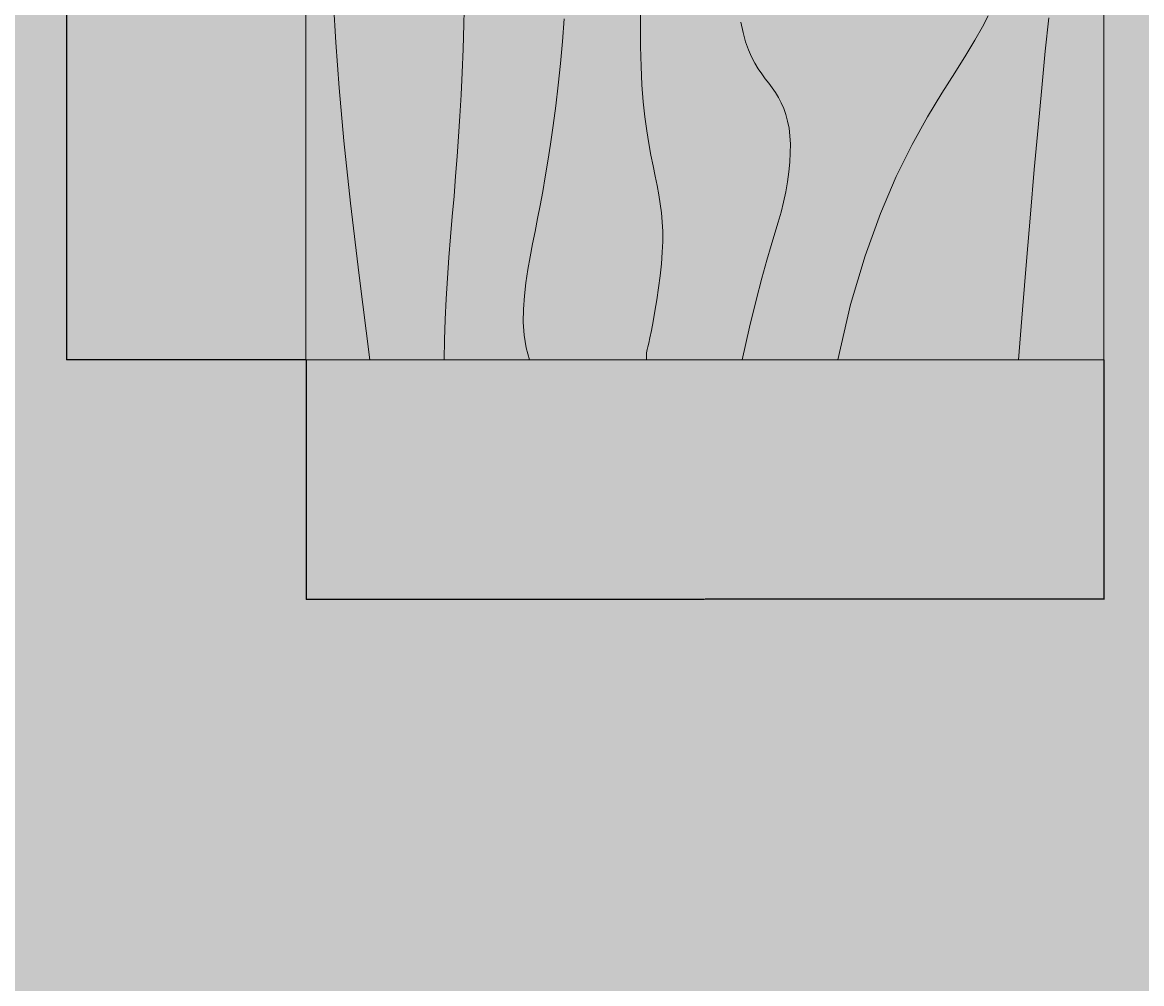
# Model space of a CAD drawing. Units: millimetres. Extents: x -229 to 16545, y -10488 to 4272.
# Tile 15 of 29: x 11804 to 12629, y -4126 to -3417. Entities that reach past the tile are written whole.
import ezdxf

# ---------------------------------------------------------------- set-up
doc = ezdxf.new("R2010")
doc.units = ezdxf.units.MM
for name, color, linetype, lineweight in [('A-ANNO-DIMS', 2, 'Continuous', 18), ('A-FURN', 8, 'Continuous', 18), ('A-FURN-PATT', 252, 'Continuous', 13)]:
    doc.layers.add(name, color=color, linetype=linetype, lineweight=lineweight)
doc.layers.add('A-FLOR-PATT', color=254, linetype='Continuous', lineweight=13, true_color=0xfeeab9)
doc.styles.get("Standard").update_dxf_attribs({"font": 'arial.ttf'})
doc.dimstyles.get("Standard").update_dxf_attribs({"dimtxt": 0.18, "dimasz": 0.18, "dimexe": 0.18, "dimexo": 0.0625, "dimgap": 0.09, "dimtad": 0, "dimtih": 1, "dimtoh": 1, "dimdec": 4, "dimzin": 0, "dimdsep": 46, "dimtxsty": 'Standard', "dimcen": 0.09, "dimadec": 0, "dimazin": 0, "dimtfac": 1, "dimtdec": 4, "dimtofl": 0, "dimtmove": 0, "dimatfit": 3, "dimfxl": 1, "dimtolj": 1, "dimtzin": 0, "dimarcsym": 0})

# ---------------------------------------------------------------- blocks, each defined once
blk = doc.blocks.new('Table - Rectangular Woodgrain 60 x 30 in.')
for p, q in [((60, 0), (0, 0)), ((60, -30), (60, 0)), ((0, -30), (60, -30))]:
    blk.add_line(p, q)
for points in [[(47.1333, -2.0667), (48.3862, -2.1947), (49.7625, -2.3281), (51.2513, -2.4663), (52.8416, -2.6083), (54.5226, -2.7535), (56.2833, -2.9011), (58.1127, -3.0501), (60, -3.2)], [(47.0542, -4.3417), (47.4756, -4.5629), (47.9661, -4.8427), (48.5372, -5.1866), (49.2, -5.6), (49.9676, -6.0844), (50.8594, -6.625), (51.8965, -7.2031), (53.1, -7.8), (54.491, -8.3969), (56.0906, -8.975), (57.9199, -9.5156), (60, -10)], [(47.2906, -13.6417), (47.6858, -13.5604), (48.0333, -13.4667), (48.3375, -13.3608), (48.6042, -13.2448), (48.8396, -13.121), (49.05, -12.9917), (49.2417, -12.8593), (49.4208, -12.7261), (49.5937, -12.5944), (49.7667, -12.4667), (49.9452, -12.3451), (50.1323, -12.2313), (50.3303, -12.1268), (50.5416, -12.0333), (50.7686, -11.9524), (51.0135, -11.8854), (51.2788, -11.8341), (51.5666, -11.8), (51.8785, -11.7843), (52.2116, -11.7865), (52.562, -11.8059), (52.926, -11.8417), (53.2998, -11.8931), (53.6795, -11.9594), (54.0614, -12.0397), (54.4416, -12.1333), (54.8223, -12.2401), (55.2293, -12.3625), (55.6942, -12.5037), (56.2489, -12.6667), (56.9251, -12.8547), (57.7545, -13.0708), (58.7689, -13.3182), (60, -13.6)], [(46.4858, -17.4012), (47.3802, -17.4156), (48.2074, -17.416), (48.9667, -17.4), (49.6583, -17.3662), (50.2872, -17.3167), (50.8595, -17.2547), (51.3812, -17.1833), (51.8584, -17.1057), (52.2971, -17.025), (52.7034, -16.9443), (53.0833, -16.8667), (53.443, -16.7951), (53.789, -16.7313), (54.128, -16.6768), (54.4666, -16.6334), (54.8115, -16.6024), (55.1693, -16.5854), (55.5465, -16.5841), (55.95, -16.6), (56.3828, -16.6337), (56.8346, -16.6823), (57.2915, -16.7418), (57.7396, -16.8084), (58.165, -16.878), (58.5539, -16.9469), (58.8924, -17.0111), (59.1666, -17.0667), (59.3679, -17.1107), (59.5078, -17.1438), (59.6032, -17.1675), (59.6708, -17.1833), (59.7275, -17.193), (59.7901, -17.1979), (59.8753, -17.1998), (60, -17.2)], [(47.1747, -20.2844), (48.0163, -20.3488), (48.8479, -20.425), (49.66, -20.5106), (50.4429, -20.6031), (51.1872, -20.7004), (51.8833, -20.8), (52.5246, -20.8999), (53.1166, -20.9995), (53.6681, -21.0983), (54.1875, -21.1958), (54.6834, -21.2919), (55.1646, -21.3859), (55.6394, -21.4777), (56.1167, -21.5667), (56.6028, -21.6515), (57.0961, -21.7266), (57.5929, -21.7852), (58.0896, -21.8208), (58.5823, -21.8268), (59.0674, -21.7964), (59.5412, -21.723), (60, -21.6)], [(46.3557, -24.0451), (47.3667, -24.0667), (48.309, -24.0947), (49.1928, -24.1287), (50.0284, -24.168), (50.826, -24.2125), (51.5959, -24.2617), (52.3483, -24.3151), (53.0935, -24.3725), (53.8417, -24.4334), (54.6009, -24.497), (55.3699, -24.561), (56.1454, -24.6226), (56.9239, -24.6792), (57.7021, -24.7279), (58.4764, -24.7662), (59.2435, -24.7911), (60, -24.8)], [(46.5843, -28.9641), (48.0579, -28.8816), (49.7666, -28.7542), (51.7629, -28.5721), (54.0989, -28.3255), (56.8272, -28.0048), (60, -27.6)]]:
    blk.add_lwpolyline(points)
blk = doc.blocks.new('*D41')
at = {"layer": 'A-ANNO-DIMS', "color": 0, "lineweight": -2, "transparency": 16777216}
for p, q in [((12012.63, -2489.42), (11836.03, -2489.42)), ((11836.21, -2489.6), (11836.21, -3077.54)), ((11836.21, -3665.84), (11836.21, -3077.9)), ((12012.63, -3666.02), (11836.03, -3666.02))]:
    blk.add_line(p, q, dxfattribs=at)
at = {"layer": 'A-ANNO-DIMS', "color": 0, "transparency": 16777216}
for points in [[(11836.18, -2489.6), (11836.24, -2489.6), (11836.21, -2489.42)], [(11836.18, -3665.84), (11836.24, -3665.84), (11836.21, -3666.02)]]:
    blk.add_solid(points, dxfattribs=at)
at = {"layer": 'Defpoints', "color": 0, "transparency": 16777216}
for p in [(12012.7, -2489.42), (11836.21, -3666.02), (12012.7, -3666.02)]:
    blk.add_point(p, dxfattribs=at)
at = {"layer": 'A-ANNO-DIMS', "color": 0, "transparency": 16777216, "insert": (11836.21, -3077.72), "char_height": 0.18, "attachment_point": 5}
blk.add_mtext('\\A1;LOW TABLE 1177', dxfattribs=at)
blk = doc.blocks.new('*D42')
at = {"layer": 'A-ANNO-DIMS', "color": 0, "lineweight": -2, "transparency": 16777216}
for p, q in [((12012.7, -3666.08), (12012.7, -3842.69)), ((12601, -3666.08), (12601, -3842.69)), ((12012.88, -3842.51), (12306.56, -3842.51)), ((12600.82, -3842.51), (12307.14, -3842.51))]:
    blk.add_line(p, q, dxfattribs=at)
at = {"layer": 'A-ANNO-DIMS', "color": 0, "transparency": 16777216}
for points in [[(12012.88, -3842.48), (12012.88, -3842.54), (12012.7, -3842.51)], [(12600.82, -3842.48), (12600.82, -3842.54), (12601, -3842.51)]]:
    blk.add_solid(points, dxfattribs=at)
at = {"layer": 'Defpoints', "color": 0, "transparency": 16777216}
for p in [(12012.7, -3666.02), (12601, -3666.02), (12601, -3842.51)]:
    blk.add_point(p, dxfattribs=at)
at = {"layer": 'A-ANNO-DIMS', "color": 0, "transparency": 16777216, "insert": (12306.85, -3842.51), "char_height": 0.18, "attachment_point": 5}
blk.add_mtext('\\A1;588', dxfattribs=at)

msp = doc.modelspace()

# ---------------------------------------------------------------- hatches: boundary and pattern name
at = {"layer": 'A-FLOR-PATT', "transparency": 33554592}
h = msp.add_hatch(color=256, dxfattribs=at)
h.dxf.hatch_style = 1
h.paths.add_polyline_path([(7975.933, -5325.772), (7943.121, -5325.772), (7943.121, -4576.49, 0.4014527), (7225.933, -5325.772, 0.4014527), (6508.746, -4576.49), (6508.746, -5325.772), (6475.933, -5325.772), (6475.933, -5438.272), (5975.933, -5438.272), (5975.933, -7267.724), (5975.933, -7438.272), (6478.619, -7438.272), (6463.448, -7355.919), (6464.88, -7356.837), (6463.849, -7358.097), (6478.619, -7438.272), (6610.327, -7438.272), (6632.656, -7409.564), (6632.525, -7406.967), (6634.208, -7407.569), (6619.273, -7426.77), (6654.466, -7438.272), (7610.517, -7438.272), (7607.41, -7421.409), (7608.842, -7422.327), (7607.812, -7423.587), (7610.517, -7438.272), (7975.933, -7438.272)])
h.paths.add_polyline_path([(13785.933, -1208.272), (9555.933, -1208.272), (9555.933, -961.785), (9705.933, -961.785), (9705.933, -918.035), (10704.976, -918.035, 0.4014527), (9705.933, 38.215), (9555.933, 38.215), (9555.933, 2021.728), (5975.933, 2021.728), (5975.933, 755.492), (5745.933, 755.492), (5745.933, 1427.266), (2918.813, 1427.266), (2918.813, -492.942), (5013.319, -492.942), (5013.319, -978.272), (5745.933, -978.272), (5745.933, -397.513), (5975.933, -397.513), (5975.933, -1208.272), (4560.933, -1208.272), (4560.933, -1265.772), (4448.433, -1265.772), (4448.433, -1298.585), (4445.933, -1298.585), (3699.151, -1298.585, 0.4014527), (4448.433, -2015.772), (4560.933, -2015.772), (4560.933, -2384.177), (5745.933, -2384.177), (5799.402, -2384.177), (5799.402, -4518.272), (5975.933, -4518.272), (5975.933, -5208.272), (6475.933, -5208.272), (6475.933, -4575.772), (6508.746, -4575.772), (6508.746, -4576.49, -0.3564726), (7216.672, -5208.272), (7235.194, -5208.272, -0.3564726), (7943.121, -4576.49), (7943.121, -4575.772), (7975.933, -4575.772), (7975.933, -5208.272), (11176.247, -5208.272), (11159.44, -5191.465), (10520.768, -5191.465), (10520.768, -4888.936), (10571.19, -4888.936), (10571.19, -4872.129), (10772.876, -4872.129), (10772.876, -4888.936), (10789.683, -4888.936), (10789.683, -4872.129), (10991.368, -4872.129), (10991.368, -4888.936), (11041.79, -4888.936), (11041.79, -4872.129), (11058.597, -4872.129, -0.0909091), (11428.354, -4872.129), (11445.162, -4872.129), (11445.162, -4888.936), (11529.197, -4888.936), (11529.197, -5191.465), (11327.512, -5191.465), (11310.704, -5208.272), (13785.933, -5208.272)])
h.paths.add_polyline_path([(11047.216, -1630.944, -1), (11402.816, -1630.944, -1)], flags=16)
h.paths.add_polyline_path([(11148.816, -1630.944), (11225.016, -1554.744), (11301.216, -1630.944), (11225.016, -1707.144)], flags=0)
h.paths.add_polyline_path([(11199.616, -1630.944, -1), (11250.416, -1630.944, -1)], flags=0)
h.paths.add_polyline_path([(11588.751, -2096.259), (11588.751, -1543.254, -0.266667), (12864.918, -1543.254), (12864.918, -2096.259), (12737.302, -2096.259), (12737.302, -2063.121), (11716.368, -2063.121), (11716.368, -2096.259)], flags=16)
h.paths.add_polyline_path([(12012.696, -2489.42), (12600.997, -2489.42), (12600.997, -3666.022), (12012.696, -3666.022)], flags=16)
h.paths.add_polyline_path([(12176.41, -3599.403), (12174.938, -3609.076), (12173.789, -3618.819), (12173.09, -3628.559), (12172.973, -3638.221), (12173.89, -3652.852), (12175.008, -3657.025), (12172.909, -3643.473), (12173.142, -3624.297), (12175.386, -3605.273)], flags=0)
h.paths.add_polyline_path([(8026.289, -286.944), (7737.703, -287.19), (7734.87, -269.156), (8029.092, -268.905)], flags=16)
h.paths.add_polyline_path([(7733.453, -260.139), (7710.784, -115.865), (7557.191, -115.996), (7556.999, 109.744), (7412.687, 132.166), (7412.433, 429.206), (7556.707, 451.876), (7556.568, 614.769), (7412.256, 637.19), (7412.003, 934.231), (7556.276, 956.9), (7556.084, 1182.639), (7709.677, 1182.77), (7732.099, 1327.082), (8029.14, 1327.335), (8051.808, 1183.062), (8205.401, 1183.192), (8205.594, 957.454), (8349.906, 935.031), (8350.159, 637.99), (8205.885, 615.322), (8206.024, 452.43), (8350.336, 430.006), (8350.59, 132.965), (8206.316, 110.298), (8206.509, -115.442), (8052.916, -115.573), (8030.493, -259.885)], flags=16)
h.paths.add_polyline_path([(12261.416, -3475.554), (12262.632, -3486.776), (12264.032, -3497.007), (12265.554, -3506.365), (12267.136, -3514.968), (12268.719, -3522.935), (12271.304, -3535.59), (12273.606, -3548.078), (12275.271, -3561.064), (12275.93, -3574.938), (12275.325, -3590.3), (12273.425, -3607.964), (12270.795, -3625.658), (12268.066, -3641.063), (12266.318, -3649.679), (12265.456, -3653.626), (12263.984, -3659.846), (12264.032, -3659.566), (12264.342, -3658.241), (12264.807, -3656.37), (12265.456, -3653.626), (12266.318, -3649.679), (12267.409, -3644.302), (12268.668, -3637.664), (12270.019, -3630.037), (12271.384, -3621.695), (12272.69, -3612.908), (12273.857, -3603.948), (12274.81, -3595.088), (12275.47, -3586.601), (12275.782, -3578.689), (12275.757, -3571.292), (12275.423, -3564.275), (12274.816, -3557.512), (12273.964, -3550.872), (12272.896, -3544.224), (12271.645, -3537.439), (12270.24, -3530.385), (12267.543, -3517.181), (12264.612, -3501.247), (12261.849, -3481.059)], flags=0)
h.paths.add_polyline_path([(12332.136, -3408.03), (12333.483, -3416.79), (12335.077, -3424.54), (12336.915, -3431.355), (12338.991, -3437.32), (12341.266, -3442.55), (12343.694, -3447.166), (12346.229, -3451.292), (12348.826, -3455.051), (12351.438, -3458.563), (12357.476, -3466.491), (12363.61, -3476.575), (12368.309, -3489.762), (12369.929, -3503.427), (12369.842, -3516.511), (12368.43, -3530.867), (12365.816, -3545.835), (12362.382, -3559.786), (12360.968, -3564.487), (12363.063, -3557.021), (12364.898, -3549.566), (12366.473, -3542.077), (12367.773, -3534.631), (12368.781, -3527.301), (12369.483, -3520.162), (12369.863, -3513.291), (12369.906, -3506.759), (12369.599, -3500.643), (12368.93, -3494.999), (12367.924, -3489.796), (12366.61, -3484.994), (12365.024, -3480.542), (12363.19, -3476.399), (12361.141, -3472.516), (12358.909, -3468.847), (12356.525, -3465.347), (12354.02, -3461.954), (12351.438, -3458.563), (12345.462, -3450.529), (12339.923, -3439.996), (12335.85, -3428.296), (12332.68, -3412.888)], flags=0)
h.paths.add_polyline_path([(12385.287, -3334.612), (12384.977, -3342.409), (12385.02, -3349.196), (12385.4, -3355.066), (12386.104, -3360.105), (12387.112, -3364.41), (12388.412, -3368.071), (12389.987, -3371.181), (12391.823, -3373.832), (12393.919, -3376.097), (12396.337, -3377.978), (12399.153, -3379.462), (12402.445, -3380.531), (12406.289, -3381.172), (12410.758, -3381.371), (12415.935, -3381.106), (12421.893, -3380.368), (12428.658, -3379.159), (12436.069, -3377.55), (12443.907, -3375.635), (12451.961, -3373.505), (12460.015, -3371.254), (12467.853, -3368.971), (12475.263, -3366.749), (12482.029, -3364.68), (12491.877, -3361.657), (12497.701, -3360.107), (12501.639, -3359.288), (12510.135, -3358.326), (12519.662, -3365.412), (12524.243, -3378.911), (12523.764, -3390.7), (12520.746, -3401.577), (12514.248, -3415.634), (12511.518, -3420.418), (12515.856, -3412.154), (12519.153, -3405.024), (12521.516, -3398.804), (12523.049, -3393.276), (12523.865, -3388.212), (12524.059, -3383.441), (12523.7, -3378.958), (12522.853, -3374.815), (12521.576, -3371.054), (12519.931, -3367.722), (12517.982, -3364.865), (12515.786, -3362.529), (12513.405, -3360.758), (12510.877, -3359.588), (12508.136, -3358.982), (12505.086, -3358.897), (12501.639, -3359.288), (12497.701, -3360.107), (12493.183, -3361.309), (12487.988, -3362.851), (12476.403, -3366.408), (12463.335, -3370.326), (12447.372, -3374.788), (12431.759, -3378.604), (12418.504, -3380.974), (12405.811, -3381.624), (12394.725, -3378.025), (12388.039, -3368.367), (12385.583, -3357.877), (12384.826, -3346.204), (12385.428, -3331.059), (12385.953, -3325.719)], flags=0)
h.paths.add_polyline_path([(7880.016, 1173.969), (7880.373, 1175.495), (7880.433, 1175.851), (7879.484, 1171.818)], flags=0)
h.paths.add_polyline_path([(7802.33, 874.962), (7800.771, 885.032), (7798.932, 893.941), (7796.811, 901.774), (7794.419, 908.63), (7791.798, 914.639), (7789.002, 919.945), (7786.083, 924.686), (7783.093, 929.005), (7780.087, 933.043), (7774.996, 939.717), (7768.406, 949.37), (7762.174, 963.427), (7759.342, 978.002), (7758.629, 991.888), (7759.492, 1007.928), (7761.801, 1025.496), (7765.392, 1044.035), (7766.625, 1049.048), (7764.522, 1039.543), (7762.719, 1030.232), (7761.232, 1021.168), (7760.08, 1012.405), (7759.28, 1003.994), (7758.849, 995.988), (7758.806, 988.44), (7759.167, 981.404), (7759.942, 974.914), (7761.104, 968.936), (7762.617, 963.414), (7764.448, 958.299), (7766.559, 953.535), (7768.918, 949.073), (7771.487, 944.856), (7774.232, 940.835), (7777.115, 936.938), (7782.377, 930.041), (7787.845, 922.139), (7793.348, 911.698), (7798.042, 898.247), (7801.702, 880.527)], flags=0)
h.paths.add_polyline_path([(12519.068, -3228.534), (12519.615, -3236.235), (12520.529, -3242.343), (12521.78, -3247.103), (12523.337, -3250.758), (12525.171, -3253.556), (12527.248, -3255.709), (12529.522, -3257.296), (12531.95, -3258.361), (12534.486, -3258.949), (12537.082, -3259.11), (12539.694, -3258.888), (12542.277, -3258.329), (12544.781, -3257.478), (12547.173, -3256.388), (12549.46, -3255.129), (12550.455, -3254.517), (12555.825, -3251.109), (12557.835, -3249.942), (12565.181, -3246.404), (12574.565, -3253.032), (12576.931, -3265.022), (12576.627, -3277.425), (12575.416, -3290.819), (12574.851, -3295.392), (12575.708, -3287.593), (12576.322, -3280.806), (12576.688, -3274.939), (12576.812, -3269.899), (12576.688, -3265.593), (12576.322, -3261.932), (12575.708, -3258.822), (12574.851, -3256.172), (12573.753, -3253.905), (12572.439, -3252.005), (12570.943, -3250.474), (12569.293, -3249.309), (12567.523, -3248.513), (12565.658, -3248.083), (12563.732, -3248.022), (12561.777, -3248.328), (12559.814, -3248.989), (12557.835, -3249.942), (12555.825, -3251.109), (12553.77, -3252.413), (12551.652, -3253.78), (12549.46, -3255.129), (12543.167, -3258.594), (12532.661, -3259.485), (12524.685, -3253.923), (12520.949, -3245.152), (12519.138, -3233.042)], flags=0)
h.paths.add_polyline_path([(7741.293, 790.501), (7741.641, 799.467), (7741.584, 807.269), (7741.141, 814.015), (7740.329, 819.809), (7739.165, 824.757), (7737.667, 828.966), (7735.853, 832.541), (7733.74, 835.586), (7731.348, 838.188), (7728.71, 840.348), (7725.861, 842.052), (7722.836, 843.28), (7719.671, 844.015), (7716.4, 844.237), (7713.06, 843.932), (7709.684, 843.081), (7706.304, 841.686), (7702.923, 839.834), (7699.543, 837.629), (7696.164, 835.178), (7692.784, 832.585), (7684.718, 826.315), (7675.609, 820.63), (7664.001, 817.274), (7654.105, 821.884), (7647.171, 832.02), (7644.191, 846.522), (7646.321, 860.288), (7647.49, 864.223), (7645.946, 857.865), (7645.046, 852.044), (7644.827, 846.557), (7645.243, 841.404), (7646.221, 836.642), (7647.693, 832.318), (7649.587, 828.489), (7651.832, 825.206), (7654.359, 822.523), (7657.097, 820.49), (7659.984, 819.145), (7662.993, 818.452), (7666.108, 818.357), (7669.311, 818.809), (7672.583, 819.755), (7675.908, 821.139), (7679.268, 822.913), (7682.645, 825.021), (7686.025, 827.401), (7689.404, 829.958), (7692.784, 832.585), (7700.505, 838.509), (7709.871, 843.64), (7721.436, 844.698), (7733.277, 837.617), (7739.571, 825.214), (7741.557, 811.049), (7741.669, 795.575)], flags=0)
h.paths.add_polyline_path([(8377.641, 137.216), (8359.607, 134.382), (8359.356, 428.605), (8377.395, 425.802)], flags=16)
h.paths.add_polyline_path([(7650.715, 668.465), (7650.08, 677.319), (7649.023, 684.34), (7647.579, 689.811), (7645.785, 694.012), (7643.675, 697.228), (7641.286, 699.7), (7638.669, 701.521), (7635.876, 702.744), (7632.96, 703.419), (7629.974, 703.601), (7626.971, 703.344), (7624.004, 702.697), (7621.125, 701.717), (7618.375, 700.462), (7615.749, 699.013), (7614.561, 698.279), (7608.435, 694.382), (7606.125, 693.04), (7598.981, 689.594), (7589.669, 693.773), (7585.26, 702.856), (7584.221, 713.11), (7584.49, 724.584), (7585.863, 739.937), (7586.518, 745.277), (7585.539, 736.31), (7584.841, 728.507), (7584.424, 721.761), (7584.288, 715.966), (7584.433, 711.016), (7584.86, 706.807), (7585.567, 703.231), (7586.556, 700.186), (7587.821, 697.58), (7589.332, 695.397), (7591.053, 693.637), (7592.951, 692.3), (7594.989, 691.385), (7597.132, 690.895), (7599.346, 690.826), (7601.594, 691.18), (7603.851, 691.943), (7606.125, 693.04), (7608.435, 694.382), (7610.797, 695.885), (7613.229, 697.458), (7620.475, 701.929), (7632.001, 704.44), (7643.476, 699.417), (7648.536, 687.571), (7650.63, 673.661)], flags=0)
h.paths.add_polyline_path([(7385.628, 136.37), (7385.382, 424.956), (7403.416, 427.789), (7403.667, 133.567)], flags=16)
h.paths.add_polyline_path([(12993.884, -2257.186), (12959.588, -2257.186), (12959.588, -2125.099), (13531.966, -2125.099, -0.1904762), (13531.966, -3974.321), (12959.588, -3974.321), (12959.588, -3842.233), (12993.884, -3842.233)], flags=16)
h.paths.add_polyline_path([(13413.486, -3313.884), (13413.486, -2785.535), (13562.885, -2785.535, -0.0496282), (13562.885, -3313.884)], flags=0)
h.paths.add_polyline_path([(8377.21, 642.241), (8359.176, 639.407), (8358.925, 933.629), (8376.964, 930.826)], flags=16)
h.paths.add_polyline_path([(13086.058, -1864.83), (13086.058, -1449.84), (13501.048, -1449.84), (13501.048, -1864.83)], flags=16)
h.paths.add_polyline_path([(13305.814, -1862.197), (13302.103, -1859.624), (13298.088, -1857.068), (13293.799, -1854.536), (13289.262, -1852.031), (13284.504, -1849.559), (13279.554, -1847.125), (13274.439, -1844.735), (13269.17, -1842.389), (13263.701, -1840.081), (13257.97, -1837.797), (13251.914, -1835.525), (13245.472, -1833.252), (13238.582, -1830.968), (13231.18, -1828.66), (13223.206, -1826.315), (13209.182, -1822.458), (13204.584, -1821.48), (13217.962, -1824.773), (13235.072, -1829.804), (13248.777, -1834.349), (13260.829, -1838.869), (13274.479, -1844.63), (13289.675, -1852.101), (13302.553, -1859.704)], flags=0)
h.paths.add_polyline_path([(13428.104, -1820.994), (13419.007, -1818.141), (13409.95, -1815.4), (13400.766, -1812.747), (13391.271, -1810.151), (13376.087, -1806.251), (13370.618, -1805.019), (13386.304, -1808.794), (13405.087, -1813.928), (13423.014, -1819.354)], flags=0)
h.paths.add_polyline_path([(7385.197, 641.395), (7384.951, 929.98), (7402.986, 932.814), (7403.236, 638.592)], flags=16)
h.paths.add_polyline_path([(13262.537, -1725.526), (13253.246, -1724.74), (13244.516, -1724.117), (13235.94, -1723.625), (13223.267, -1723.062), (13217.598, -1722.912), (13231.966, -1723.397), (13248.733, -1724.359), (13266.899, -1725.895), (13272.802, -1726.502)], flags=0)
h.paths.add_polyline_path([(13191.893, -1641.137), (13208.675, -1640.506), (13214.057, -1640.258), (13197.763, -1640.936)], flags=0)
h.paths.add_polyline_path([(13097.524, -1608.457), (13114.284, -1609.031), (13120.126, -1609.105), (13103.045, -1608.71)], flags=0)
h.paths.add_polyline_path([(13465.328, -1521.577), (13473.906, -1517.015), (13481.761, -1511.636), (13492.562, -1502.076), (13495.327, -1497.933), (13485.818, -1508.858), (13470.208, -1519.547)], flags=0)
h.paths.add_polyline_path([(13175.015, -1500.891), (13184.046, -1501.807), (13192.721, -1502.52), (13201.114, -1503.034), (13209.273, -1503.351), (13217.244, -1503.476), (13225.078, -1503.41), (13232.821, -1503.16), (13240.524, -1502.728), (13248.233, -1502.117), (13255.993, -1501.322), (13263.825, -1500.293), (13271.746, -1498.974), (13279.775, -1497.305), (13287.928, -1495.229), (13296.222, -1492.688), (13304.675, -1489.622), (13313.304, -1485.975), (13322.089, -1481.727), (13330.859, -1477.028), (13339.408, -1472.063), (13347.526, -1467.02), (13355.006, -1462.087), (13364.86, -1455.202), (13367.224, -1453.299), (13358.544, -1459.754), (13343.348, -1469.775), (13326.143, -1479.767), (13309.023, -1488.045), (13292.249, -1494.129), (13276.009, -1498.264), (13260.299, -1500.88), (13244.401, -1502.51), (13228.945, -1503.378), (13213.316, -1503.508), (13197.047, -1502.876), (13180.088, -1501.481)], flags=0)
h.paths.add_polyline_path([(7733.501, 1336.101), (7736.303, 1354.14), (8024.889, 1354.386), (8027.723, 1336.352)], flags=16)
at = {"layer": 'A-FURN-PATT', "transparency": 33554569}
h = msp.add_hatch(color=256, dxfattribs=at)
h.dxf.hatch_style = 1
h.paths.add_polyline_path([(12600.997, -2489.42), (12553.933, -2489.42), (12553.58, -2583.852), (12552.584, -2666.503), (12551.036, -2738.644), (12549.03, -2801.547), (12546.656, -2856.483), (12544.004, -2904.723), (12541.171, -2947.542), (12538.245, -2986.207), (12535.313, -3021.787), (12532.444, -3054.526), (12529.695, -3084.461), (12527.132, -3111.629), (12524.814, -3136.073), (12522.802, -3157.826), (12521.157, -3176.928), (12519.941, -3193.42), (12519.202, -3207.371), (12518.921, -3218.994), (12519.068, -3228.534), (12519.615, -3236.235), (12520.529, -3242.343), (12521.78, -3247.103), (12523.337, -3250.758), (12525.171, -3253.556), (12527.248, -3255.709), (12529.522, -3257.296), (12531.95, -3258.361), (12534.486, -3258.949), (12537.082, -3259.11), (12539.694, -3258.888), (12542.277, -3258.329), (12544.781, -3257.478), (12547.173, -3256.388), (12549.46, -3255.129), (12551.652, -3253.78), (12559.563, -3248.675), (12566.794, -3247.543), (12572.687, -3251.706), (12575.978, -3258.498), (12576.872, -3267.431), (12576.627, -3277.425), (12575.708, -3287.593), (12574.851, -3295.392), (12573.749, -3304.309), (12572.419, -3314.522), (12570.874, -3326.221), (12569.131, -3339.597), (12567.203, -3354.842), (12565.107, -3372.146), (12562.857, -3391.705), (12560.469, -3413.705), (12557.959, -3438.275), (12555.343, -3465.264), (12552.633, -3494.46), (12549.848, -3525.645), (12547.001, -3558.61), (12544.106, -3593.137), (12541.184, -3629.012), (12538.245, -3666.022), (12600.997, -3666.022)])
h.paths.add_polyline_path([(12544.004, -2904.723), (12546.656, -2856.483), (12549.03, -2801.547), (12551.036, -2738.644), (12552.584, -2666.503), (12553.58, -2583.852), (12553.933, -2489.42), (12420.585, -2489.42), (12422.824, -2618.374), (12423.791, -2723.534), (12423.687, -2808.136), (12422.708, -2875.41), (12421.057, -2928.591), (12418.93, -2970.907), (12416.527, -3005.595), (12414.049, -3035.885), (12411.656, -3064.467), (12409.37, -3091.846), (12407.177, -3117.984), (12405.059, -3142.842), (12403.004, -3166.384), (12400.994, -3188.569), (12399.016, -3209.359), (12397.053, -3228.718), (12395.1, -3246.62), (12393.191, -3263.097), (12391.376, -3278.194), (12389.699, -3291.961), (12388.205, -3304.438), (12386.942, -3315.677), (12385.953, -3325.719), (12385.287, -3334.612), (12384.977, -3342.409), (12385.02, -3349.196), (12385.4, -3355.066), (12386.104, -3360.105), (12387.112, -3364.41), (12388.412, -3368.071), (12389.987, -3371.181), (12391.823, -3373.832), (12393.919, -3376.097), (12396.337, -3377.978), (12399.153, -3379.462), (12402.445, -3380.531), (12406.289, -3381.172), (12410.758, -3381.371), (12415.935, -3381.106), (12421.893, -3380.368), (12428.658, -3379.159), (12436.069, -3377.55), (12443.907, -3375.635), (12451.961, -3373.505), (12460.015, -3371.254), (12467.853, -3368.971), (12475.263, -3366.749), (12482.029, -3364.68), (12491.877, -3361.657), (12502.516, -3358.826), (12511.128, -3359.064), (12517.01, -3363.44), (12520.955, -3369.223), (12523.527, -3376.802), (12524.25, -3385.824), (12522.632, -3395.865), (12519.153, -3405.024), (12515.856, -3412.154), (12511.518, -3420.418), (12506.031, -3430.037), (12499.288, -3441.236), (12491.181, -3454.234), (12481.682, -3469.286), (12471.081, -3486.774), (12459.744, -3507.112), (12448.039, -3530.713), (12436.334, -3557.99), (12424.997, -3589.358), (12414.396, -3625.231), (12404.897, -3666.022), (12538.245, -3666.022), (12541.184, -3629.012), (12544.106, -3593.137), (12547.001, -3558.61), (12549.848, -3525.645), (12552.633, -3494.46), (12555.343, -3465.264), (12557.959, -3438.275), (12560.469, -3413.705), (12562.857, -3391.705), (12565.107, -3372.146), (12567.203, -3354.842), (12569.131, -3339.597), (12570.874, -3326.221), (12572.419, -3314.522), (12573.749, -3304.309), (12574.851, -3295.392), (12575.708, -3287.593), (12576.322, -3280.806), (12576.688, -3274.939), (12576.812, -3269.899), (12576.688, -3265.593), (12576.322, -3261.932), (12575.708, -3258.822), (12574.851, -3256.172), (12573.753, -3253.905), (12572.439, -3252.005), (12570.943, -3250.474), (12569.293, -3249.309), (12567.523, -3248.513), (12565.658, -3248.083), (12563.732, -3248.022), (12561.777, -3248.328), (12559.814, -3248.989), (12557.835, -3249.942), (12555.825, -3251.109), (12553.77, -3252.413), (12547.19, -3256.659), (12539.533, -3259.262), (12531.64, -3258.773), (12524.685, -3253.923), (12520.949, -3245.152), (12519.615, -3236.235), (12519.068, -3228.534), (12518.921, -3218.994), (12519.202, -3207.371), (12519.941, -3193.42), (12521.157, -3176.928), (12522.802, -3157.826), (12524.814, -3136.073), (12527.132, -3111.629), (12529.695, -3084.461), (12532.444, -3054.526), (12535.313, -3021.787), (12538.245, -2986.207), (12541.171, -2947.542)])
h.paths.add_polyline_path([(12418.93, -2970.907), (12421.057, -2928.591), (12422.708, -2875.41), (12423.687, -2808.136), (12423.791, -2723.534), (12422.824, -2618.374), (12420.585, -2489.42), (12349.989, -2489.42), (12347.396, -2591.092), (12345.433, -2678.094), (12343.99, -2752.122), (12342.962, -2814.864), (12342.239, -2868.017), (12341.715, -2913.271), (12341.284, -2952.323), (12340.837, -2986.86), (12340.288, -3018.358), (12339.633, -3047.386), (12338.883, -3074.301), (12338.06, -3099.455), (12337.173, -3123.199), (12336.242, -3145.885), (12335.279, -3167.868), (12334.301, -3189.498), (12333.326, -3211.038), (12332.381, -3232.395), (12331.496, -3253.384), (12330.706, -3273.821), (12330.037, -3293.523), (12329.52, -3312.306), (12329.188, -3329.984), (12329.071, -3346.378), (12329.194, -3361.343), (12329.561, -3374.915), (12330.175, -3387.169), (12331.032, -3398.18), (12332.136, -3408.03), (12333.483, -3416.79), (12335.077, -3424.54), (12336.915, -3431.355), (12338.991, -3437.32), (12341.266, -3442.55), (12343.694, -3447.166), (12346.229, -3451.292), (12348.826, -3455.051), (12351.438, -3458.563), (12357.476, -3466.491), (12362.356, -3474.514), (12365.989, -3482.725), (12368.611, -3492.308), (12369.929, -3503.427), (12369.863, -3513.291), (12369.483, -3520.162), (12368.781, -3527.301), (12367.773, -3534.631), (12366.473, -3542.077), (12364.898, -3549.566), (12363.063, -3557.021), (12360.968, -3564.487), (12358.568, -3572.468), (12355.799, -3581.585), (12352.603, -3592.463), (12348.916, -3605.723), (12344.678, -3621.988), (12339.827, -3641.88), (12334.301, -3666.022), (12404.897, -3666.022), (12414.396, -3625.231), (12424.997, -3589.358), (12436.334, -3557.99), (12448.039, -3530.713), (12459.744, -3507.112), (12471.081, -3486.774), (12481.682, -3469.286), (12491.181, -3454.234), (12499.288, -3441.236), (12506.031, -3430.037), (12511.518, -3420.418), (12515.856, -3412.154), (12519.153, -3405.024), (12521.516, -3398.804), (12523.049, -3393.276), (12523.865, -3388.212), (12524.059, -3383.441), (12523.7, -3378.958), (12522.853, -3374.815), (12521.576, -3371.054), (12519.931, -3367.722), (12517.982, -3364.865), (12515.786, -3362.529), (12513.405, -3360.758), (12510.877, -3359.588), (12508.136, -3358.982), (12505.086, -3358.897), (12501.639, -3359.288), (12497.701, -3360.107), (12493.183, -3361.309), (12487.988, -3362.851), (12476.403, -3366.408), (12463.335, -3370.326), (12451.961, -3373.505), (12439.372, -3376.834), (12424.661, -3380.026), (12412.995, -3381.47), (12402.039, -3380.984), (12393.748, -3376.613), (12389.022, -3369.787), (12386.442, -3362.522), (12385.041, -3352.492), (12384.977, -3342.409), (12385.287, -3334.612), (12385.953, -3325.719), (12386.942, -3315.677), (12388.205, -3304.438), (12389.699, -3291.961), (12391.376, -3278.194), (12393.191, -3263.097), (12395.1, -3246.62), (12397.053, -3228.718), (12399.016, -3209.359), (12400.994, -3188.569), (12403.004, -3166.384), (12405.059, -3142.842), (12407.177, -3117.984), (12409.37, -3091.846), (12411.656, -3064.467), (12414.049, -3035.885), (12416.527, -3005.595)])
h.paths.add_polyline_path([(12340.837, -2986.86), (12341.284, -2952.323), (12341.715, -2913.271), (12342.239, -2868.017), (12342.962, -2814.864), (12343.99, -2752.122), (12345.433, -2678.094), (12347.396, -2591.092), (12349.989, -2489.42), (12248.016, -2489.42), (12253.364, -2589.902), (12257.71, -2678.871), (12261.149, -2757.499), (12263.787, -2826.958), (12265.718, -2888.42), (12267.044, -2943.055), (12267.866, -2992.039), (12268.279, -3036.54), (12268.378, -3077.58), (12268.209, -3115.572), (12267.809, -3150.776), (12267.219, -3183.452), (12266.473, -3213.86), (12265.614, -3242.261), (12264.679, -3268.917), (12263.704, -3294.084), (12262.732, -3317.981), (12261.804, -3340.639), (12260.969, -3362.039), (12260.273, -3382.167), (12259.759, -3401.008), (12259.477, -3418.547), (12259.469, -3434.769), (12259.782, -3449.659), (12260.445, -3463.221), (12261.416, -3475.554), (12262.632, -3486.776), (12264.032, -3497.007), (12265.554, -3506.365), (12267.136, -3514.968), (12268.719, -3522.935), (12271.304, -3535.59), (12273.606, -3548.078), (12275.271, -3561.064), (12275.757, -3571.292), (12275.782, -3578.689), (12275.47, -3586.601), (12274.81, -3595.088), (12273.857, -3603.948), (12272.69, -3612.908), (12271.384, -3621.695), (12270.019, -3630.037), (12268.066, -3641.063), (12265.651, -3652.97), (12264.342, -3658.241), (12264.032, -3659.566), (12263.842, -3660.678), (12263.746, -3661.906), (12263.708, -3663.576), (12263.704, -3666.022), (12334.301, -3666.022), (12339.827, -3641.88), (12344.678, -3621.988), (12348.916, -3605.723), (12352.603, -3592.463), (12355.799, -3581.585), (12358.568, -3572.468), (12360.968, -3564.487), (12363.063, -3557.021), (12364.898, -3549.566), (12366.473, -3542.077), (12367.773, -3534.631), (12368.781, -3527.301), (12369.483, -3520.162), (12369.863, -3513.291), (12369.906, -3506.759), (12369.599, -3500.643), (12368.93, -3494.999), (12367.924, -3489.796), (12366.61, -3484.994), (12365.024, -3480.542), (12363.19, -3476.399), (12361.141, -3472.516), (12358.909, -3468.847), (12356.525, -3465.347), (12354.02, -3461.954), (12347.609, -3453.536), (12342.257, -3444.828), (12337.759, -3434.488), (12335.077, -3424.54), (12333.483, -3416.79), (12332.136, -3408.03), (12331.032, -3398.18), (12330.175, -3387.169), (12329.561, -3374.915), (12329.194, -3361.343), (12329.071, -3346.378), (12329.188, -3329.984), (12329.52, -3312.306), (12330.037, -3293.523), (12330.706, -3273.821), (12331.496, -3253.384), (12332.381, -3232.395), (12333.326, -3211.038), (12334.301, -3189.498), (12335.279, -3167.868), (12336.242, -3145.885), (12337.173, -3123.199), (12338.06, -3099.455), (12338.883, -3074.301), (12339.633, -3047.386), (12340.288, -3018.358)])
h.paths.add_polyline_path([(12267.866, -2992.039), (12267.044, -2943.055), (12265.718, -2888.42), (12263.787, -2826.958), (12261.149, -2757.499), (12257.71, -2678.871), (12253.364, -2589.902), (12248.016, -2489.42), (12161.732, -2489.42), (12164.672, -2646.493), (12167.594, -2771.989), (12170.488, -2870.184), (12173.336, -2945.353), (12176.12, -3001.769), (12178.83, -3043.709), (12181.446, -3075.446), (12183.956, -3101.253), (12186.347, -3124.72), (12188.614, -3146.693), (12190.759, -3167.333), (12192.781, -3186.802), (12194.681, -3205.259), (12196.458, -3222.865), (12198.113, -3239.782), (12199.644, -3256.172), (12201.048, -3272.182), (12202.3, -3287.915), (12203.368, -3303.466), (12204.221, -3318.924), (12204.827, -3334.383), (12205.161, -3349.932), (12205.186, -3365.667), (12204.874, -3381.676), (12204.208, -3398.008), (12203.219, -3414.517), (12201.956, -3431.021), (12200.462, -3447.329), (12198.784, -3463.254), (12196.97, -3478.607), (12195.062, -3493.203), (12193.108, -3506.853), (12191.149, -3519.429), (12189.196, -3531.038), (12187.259, -3541.853), (12185.347, -3552.039), (12183.462, -3561.763), (12181.619, -3571.2), (12179.819, -3580.51), (12178.073, -3589.87), (12176.41, -3599.403), (12174.938, -3609.076), (12173.789, -3618.819), (12173.09, -3628.559), (12172.973, -3638.221), (12173.569, -3647.734), (12175.008, -3657.025), (12177.42, -3666.022), (12263.654, -3666.022), (12263.777, -3660.515), (12264.807, -3656.37), (12265.456, -3653.626), (12266.318, -3649.679), (12267.409, -3644.302), (12268.668, -3637.664), (12270.019, -3630.037), (12271.384, -3621.695), (12272.69, -3612.908), (12273.857, -3603.948), (12274.81, -3595.088), (12275.47, -3586.601), (12275.782, -3578.689), (12275.757, -3571.292), (12275.423, -3564.275), (12274.816, -3557.512), (12273.964, -3550.872), (12272.896, -3544.224), (12271.645, -3537.439), (12270.24, -3530.385), (12267.543, -3517.181), (12265.554, -3506.365), (12264.032, -3497.007), (12262.632, -3486.776), (12261.416, -3475.554), (12260.445, -3463.221), (12259.782, -3449.659), (12259.469, -3434.769), (12259.477, -3418.547), (12259.759, -3401.008), (12260.273, -3382.167), (12260.969, -3362.039), (12261.804, -3340.639), (12262.732, -3317.981), (12263.704, -3294.084), (12264.679, -3268.917), (12265.614, -3242.261), (12266.473, -3213.86), (12267.219, -3183.452), (12267.809, -3150.776), (12268.209, -3115.572), (12268.378, -3077.58), (12268.279, -3036.54)])
h.paths.add_polyline_path([(12178.83, -3043.709), (12176.12, -3001.769), (12173.336, -2945.353), (12170.488, -2870.184), (12167.594, -2771.989), (12164.672, -2646.493), (12161.732, -2489.42), (12106.824, -2489.42), (12109.758, -2658.763), (12112.646, -2797.349), (12115.441, -2909.171), (12118.1, -2998.218), (12120.575, -3068.485), (12122.818, -3123.958), (12124.787, -3168.631), (12126.434, -3206.494), (12127.727, -3240.902), (12128.682, -3272.678), (12129.331, -3302.001), (12129.703, -3329.057), (12129.831, -3354.028), (12129.742, -3377.101), (12129.472, -3398.457), (12129.048, -3418.282), (12128.499, -3436.761), (12127.832, -3454.092), (12127.062, -3470.478), (12126.189, -3486.119), (12125.224, -3501.217), (12124.177, -3515.972), (12123.052, -3530.585), (12121.857, -3545.257), (12120.61, -3560.145), (12119.355, -3575.225), (12118.147, -3590.433), (12117.037, -3605.699), (12116.082, -3620.96), (12115.331, -3636.144), (12114.843, -3651.187), (12114.668, -3666.022), (12177.42, -3666.022), (12175.008, -3657.025), (12173.569, -3647.734), (12172.973, -3638.221), (12173.09, -3628.559), (12173.789, -3618.819), (12174.938, -3609.076), (12176.41, -3599.403), (12178.073, -3589.87), (12179.819, -3580.51), (12181.619, -3571.2), (12183.462, -3561.763), (12185.347, -3552.039), (12187.259, -3541.853), (12189.196, -3531.038), (12191.149, -3519.429), (12193.108, -3506.853), (12195.062, -3493.203), (12196.97, -3478.607), (12198.784, -3463.254), (12200.462, -3447.329), (12201.956, -3431.021), (12203.219, -3414.517), (12204.208, -3398.008), (12204.874, -3381.676), (12205.186, -3365.667), (12205.161, -3349.932), (12204.827, -3334.383), (12204.221, -3318.924), (12203.368, -3303.466), (12202.3, -3287.915), (12201.048, -3272.182), (12199.644, -3256.172), (12198.113, -3239.782), (12196.458, -3222.865), (12194.681, -3205.259), (12192.781, -3186.802), (12190.759, -3167.333), (12188.614, -3146.693), (12186.347, -3124.72), (12183.956, -3101.253), (12181.446, -3075.446)])
h.paths.add_polyline_path([(12120.575, -3068.485), (12118.1, -2998.218), (12115.441, -2909.171), (12112.646, -2797.349), (12109.758, -2658.763), (12106.824, -2489.42), (12036.228, -2489.42), (12038.815, -2600.936), (12040.742, -2694.345), (12042.088, -2771.942), (12042.927, -2836.027), (12043.339, -2888.898), (12043.398, -2932.852), (12043.18, -2970.187), (12042.764, -3003.203), (12042.215, -3033.834), (12041.56, -3062.574), (12040.811, -3089.552), (12039.985, -3114.898), (12039.101, -3138.743), (12038.168, -3161.217), (12037.207, -3182.448), (12036.228, -3202.57), (12035.254, -3221.743), (12034.318, -3240.249), (12033.459, -3258.402), (12032.714, -3276.518), (12032.124, -3294.908), (12031.724, -3313.888), (12031.553, -3333.773), (12031.653, -3354.875), (12032.083, -3377.629), (12033.01, -3402.94), (12034.628, -3431.837), (12037.126, -3465.345), (12040.697, -3504.492), (12045.533, -3550.301), (12051.822, -3603.803), (12059.76, -3666.022), (12114.668, -3666.022), (12114.843, -3651.187), (12115.331, -3636.144), (12116.082, -3620.96), (12117.037, -3605.699), (12118.147, -3590.433), (12119.355, -3575.225), (12120.61, -3560.145), (12121.857, -3545.257), (12123.052, -3530.585), (12124.177, -3515.972), (12125.224, -3501.217), (12126.189, -3486.119), (12127.062, -3470.478), (12127.832, -3454.092), (12128.499, -3436.761), (12129.048, -3418.282), (12129.472, -3398.457), (12129.742, -3377.101), (12129.831, -3354.028), (12129.703, -3329.057), (12129.331, -3302.001), (12128.682, -3272.678), (12127.727, -3240.902), (12126.434, -3206.494), (12124.787, -3168.631), (12122.818, -3123.958)])
h.paths.add_polyline_path([(12042.215, -3033.834), (12042.764, -3003.203), (12043.18, -2970.187), (12043.398, -2932.852), (12043.339, -2888.898), (12042.927, -2836.027), (12042.088, -2771.942), (12040.742, -2694.345), (12038.815, -2600.936), (12036.228, -2489.42), (12012.696, -2489.42), (12012.696, -3666.022), (12059.76, -3666.022), (12051.822, -3603.803), (12045.533, -3550.301), (12040.697, -3504.492), (12037.126, -3465.345), (12034.628, -3431.837), (12033.01, -3402.94), (12032.083, -3377.629), (12031.653, -3354.875), (12031.553, -3333.773), (12031.724, -3313.888), (12032.124, -3294.908), (12032.714, -3276.518), (12033.459, -3258.402), (12034.318, -3240.249), (12035.254, -3221.743), (12036.228, -3202.57), (12037.207, -3182.448), (12038.168, -3161.217), (12039.101, -3138.743), (12039.985, -3114.898), (12040.811, -3089.552), (12041.56, -3062.574)])
h.paths.add_polyline_path([(13347.526, -1467.02), (13355.006, -1462.087), (13361.641, -1457.451), (13367.224, -1453.299), (13371.521, -1449.84), (13086.058, -1449.84), (13086.058, -1489.363), (13102.895, -1491.509), (13118.03, -1493.501), (13131.658, -1495.331), (13143.974, -1496.992), (13155.175, -1498.477), (13165.457, -1499.778), (13175.015, -1500.891), (13184.046, -1501.807), (13192.721, -1502.52), (13201.114, -1503.034), (13209.273, -1503.351), (13217.244, -1503.476), (13225.078, -1503.41), (13232.821, -1503.16), (13240.524, -1502.728), (13248.233, -1502.117), (13255.993, -1501.322), (13263.825, -1500.293), (13271.746, -1498.974), (13279.775, -1497.305), (13287.928, -1495.229), (13296.222, -1492.688), (13304.675, -1489.622), (13313.304, -1485.975), (13322.089, -1481.727), (13330.859, -1477.028), (13339.408, -1472.063)], flags=17)
h.paths.add_polyline_path([(13481.761, -1511.636), (13488.9, -1505.317), (13495.327, -1497.933), (13501.048, -1489.363), (13501.048, -1449.84), (13371.521, -1449.84), (13367.224, -1453.299), (13361.641, -1457.451), (13355.006, -1462.087), (13347.526, -1467.02), (13339.408, -1472.063), (13330.859, -1477.028), (13322.089, -1481.727), (13313.304, -1485.975), (13304.675, -1489.622), (13296.222, -1492.688), (13287.928, -1495.229), (13279.775, -1497.305), (13271.746, -1498.974), (13263.825, -1500.293), (13255.993, -1501.322), (13248.233, -1502.117), (13240.524, -1502.728), (13232.821, -1503.16), (13225.078, -1503.41), (13217.244, -1503.476), (13209.273, -1503.351), (13201.114, -1503.034), (13192.721, -1502.52), (13184.046, -1501.807), (13175.015, -1500.891), (13165.457, -1499.778), (13155.175, -1498.477), (13143.974, -1496.992), (13131.658, -1495.331), (13118.03, -1493.501), (13102.895, -1491.509), (13086.058, -1489.363), (13086.058, -1528.886), (13104.044, -1529.875), (13122.361, -1531.009), (13140.808, -1532.253), (13159.186, -1533.57), (13177.296, -1534.925), (13194.937, -1536.281), (13211.91, -1537.602), (13228.015, -1538.852), (13243.116, -1539.998), (13257.327, -1541.017), (13270.825, -1541.888), (13283.787, -1542.59), (13296.39, -1543.103), (13308.811, -1543.407), (13321.227, -1543.48), (13333.816, -1543.302), (13346.703, -1542.854), (13359.802, -1542.129), (13372.977, -1541.12), (13386.091, -1539.822), (13399.008, -1538.228), (13411.589, -1536.331), (13423.699, -1534.127), (13435.201, -1531.609), (13445.981, -1528.75), (13456.022, -1525.448), (13465.328, -1521.577), (13473.906, -1517.015)])
h.paths.add_polyline_path([(13473.169, -1576.927), (13501.048, -1568.409), (13501.048, -1489.363), (13495.327, -1497.933), (13488.9, -1505.317), (13481.761, -1511.636), (13473.906, -1517.015), (13465.328, -1521.577), (13456.022, -1525.448), (13445.981, -1528.75), (13435.201, -1531.609), (13423.699, -1534.127), (13411.589, -1536.331), (13399.008, -1538.228), (13386.091, -1539.822), (13372.977, -1541.12), (13359.802, -1542.129), (13346.703, -1542.854), (13333.816, -1543.302), (13321.227, -1543.48), (13308.811, -1543.407), (13296.39, -1543.103), (13283.787, -1542.59), (13270.825, -1541.888), (13257.327, -1541.017), (13243.116, -1539.998), (13228.015, -1538.852), (13211.91, -1537.602), (13194.937, -1536.281), (13177.296, -1534.925), (13159.186, -1533.57), (13140.808, -1532.253), (13122.361, -1531.009), (13104.044, -1529.875), (13086.058, -1528.886), (13086.058, -1607.932), (13097.524, -1608.457), (13108.847, -1608.845), (13120.126, -1609.105), (13131.46, -1609.251), (13142.948, -1609.292), (13154.691, -1609.241), (13166.786, -1609.108), (13179.335, -1608.907), (13192.433, -1608.641), (13206.166, -1608.296), (13220.617, -1607.849), (13235.868, -1607.277), (13252.002, -1606.56), (13269.102, -1605.677), (13287.251, -1604.604), (13306.532, -1603.319), (13327.007, -1601.774), (13348.658, -1599.805), (13371.445, -1597.222), (13395.329, -1593.833), (13420.269, -1589.449), (13446.229, -1583.876)])
h.paths.add_polyline_path([(13501.048, -1607.932), (13458.096, -1615.209), (13420.819, -1621.063), (13388.585, -1625.678), (13360.757, -1629.235), (13336.7, -1631.917), (13315.782, -1633.906), (13297.366, -1635.385), (13280.818, -1636.535), (13265.584, -1637.513), (13251.437, -1638.359), (13238.231, -1639.089), (13225.82, -1639.718), (13214.057, -1640.258), (13202.797, -1640.727), (13191.893, -1641.137), (13181.2, -1641.502), (13170.572, -1641.845), (13159.867, -1642.207), (13148.942, -1642.635), (13137.655, -1643.178), (13125.865, -1643.884), (13113.431, -1644.799), (13100.208, -1645.973), (13086.058, -1647.454), (13086.058, -1686.977), (13124.833, -1683.82), (13159.932, -1681.185), (13191.674, -1679.027), (13220.38, -1677.299), (13246.37, -1675.957), (13269.963, -1674.954), (13291.481, -1674.247), (13311.243, -1673.788), (13329.68, -1673.559), (13347.664, -1673.645), (13366.176, -1674.156), (13386.201, -1675.203), (13408.718, -1676.899), (13434.71, -1679.352), (13465.16, -1682.674), (13501.048, -1686.977)])
h.paths.add_polyline_path([(13501.048, -1686.977), (13465.16, -1682.674), (13434.71, -1679.352), (13408.718, -1676.899), (13386.201, -1675.203), (13366.176, -1674.156), (13347.664, -1673.645), (13329.68, -1673.559), (13311.243, -1673.788), (13291.481, -1674.247), (13269.963, -1674.954), (13246.37, -1675.957), (13220.38, -1677.299), (13191.674, -1679.027), (13159.932, -1681.185), (13124.833, -1683.82), (13086.058, -1686.977), (13086.058, -1726.5), (13102.94, -1724.807), (13119.714, -1723.593), (13136.181, -1722.793), (13152.144, -1722.337), (13167.406, -1722.161), (13181.77, -1722.195), (13195.037, -1722.374), (13207.013, -1722.63), (13217.598, -1722.912), (13227.103, -1723.233), (13235.94, -1723.625), (13244.516, -1724.117), (13253.246, -1724.74), (13262.537, -1725.526), (13272.802, -1726.502), (13284.449, -1727.701), (13297.939, -1729.184), (13313.919, -1731.151), (13333.085, -1733.832), (13356.132, -1737.458), (13383.755, -1742.259), (13416.652, -1748.466), (13455.518, -1756.31), (13501.048, -1766.023)])
h.paths.add_polyline_path([(13420.819, -1621.063), (13458.096, -1615.209), (13501.048, -1607.932), (13501.048, -1568.409), (13473.169, -1576.927), (13446.229, -1583.876), (13420.269, -1589.449), (13395.329, -1593.833), (13371.445, -1597.222), (13348.658, -1599.805), (13327.007, -1601.774), (13306.532, -1603.319), (13287.251, -1604.604), (13269.102, -1605.677), (13252.002, -1606.56), (13235.868, -1607.277), (13220.617, -1607.849), (13206.166, -1608.296), (13192.433, -1608.641), (13179.335, -1608.907), (13166.786, -1609.108), (13154.691, -1609.241), (13142.948, -1609.292), (13131.46, -1609.251), (13120.126, -1609.105), (13108.847, -1608.845), (13097.524, -1608.457), (13086.058, -1607.932), (13086.058, -1647.454), (13100.208, -1645.973), (13113.431, -1644.799), (13125.865, -1643.884), (13137.655, -1643.178), (13148.942, -1642.635), (13159.867, -1642.207), (13170.572, -1641.845), (13181.2, -1641.502), (13191.893, -1641.137), (13202.797, -1640.727), (13214.057, -1640.258), (13225.82, -1639.718), (13238.231, -1639.089), (13251.437, -1638.359), (13265.584, -1637.513), (13280.818, -1636.535), (13297.366, -1635.385), (13315.782, -1633.906), (13336.7, -1631.917), (13360.757, -1629.235), (13388.585, -1625.678)])
h.paths.add_polyline_path([(13356.132, -1737.458), (13333.085, -1733.832), (13313.919, -1731.151), (13297.939, -1729.184), (13284.449, -1727.701), (13272.802, -1726.502), (13262.537, -1725.526), (13253.246, -1724.74), (13244.516, -1724.117), (13235.94, -1723.625), (13227.103, -1723.233), (13217.598, -1722.912), (13207.013, -1722.63), (13195.037, -1722.374), (13181.77, -1722.195), (13167.406, -1722.161), (13152.144, -1722.337), (13136.181, -1722.793), (13119.714, -1723.593), (13102.94, -1724.807), (13086.058, -1726.5), (13086.058, -1766.023), (13139.44, -1771.317), (13184.365, -1776.092), (13221.843, -1780.403), (13252.878, -1784.307), (13278.478, -1787.865), (13299.651, -1791.133), (13317.401, -1794.169), (13332.737, -1797.031), (13346.528, -1799.772), (13359.094, -1802.425), (13370.618, -1805.019), (13381.282, -1807.585), (13391.271, -1810.151), (13400.766, -1812.747), (13409.95, -1815.4), (13419.007, -1818.141), (13428.104, -1820.994), (13437.348, -1823.975), (13446.831, -1827.091), (13456.644, -1830.354), (13466.882, -1833.773), (13477.633, -1837.359), (13488.991, -1841.121), (13501.048, -1845.069), (13501.048, -1766.023), (13455.518, -1756.31), (13416.652, -1748.466), (13383.755, -1742.259)])
h.paths.add_polyline_path([(13299.651, -1791.133), (13278.478, -1787.865), (13252.878, -1784.307), (13221.843, -1780.403), (13184.365, -1776.092), (13139.44, -1771.317), (13086.058, -1766.023), (13086.058, -1805.546), (13115.797, -1808.369), (13140.752, -1811.122), (13161.515, -1813.805), (13178.68, -1816.424), (13192.839, -1818.981), (13204.584, -1821.48), (13214.509, -1823.923), (13223.206, -1826.315), (13231.18, -1828.66), (13238.582, -1830.968), (13245.472, -1833.252), (13251.914, -1835.525), (13257.97, -1837.797), (13263.701, -1840.081), (13269.17, -1842.389), (13274.439, -1844.735), (13279.554, -1847.125), (13284.504, -1849.559), (13289.262, -1852.031), (13293.799, -1854.536), (13298.088, -1857.068), (13302.103, -1859.624), (13305.814, -1862.197), (13309.259, -1864.83), (13501.048, -1864.83), (13501.048, -1845.069), (13488.991, -1841.121), (13477.633, -1837.359), (13466.882, -1833.773), (13456.644, -1830.354), (13446.831, -1827.091), (13437.348, -1823.975), (13428.104, -1820.994), (13419.007, -1818.141), (13409.95, -1815.4), (13400.766, -1812.747), (13391.271, -1810.151), (13381.282, -1807.585), (13370.618, -1805.019), (13359.094, -1802.425), (13346.528, -1799.772), (13332.737, -1797.031), (13317.401, -1794.169)])
h.paths.add_polyline_path([(13245.472, -1833.252), (13238.582, -1830.968), (13231.18, -1828.66), (13223.206, -1826.315), (13214.509, -1823.923), (13204.584, -1821.48), (13192.839, -1818.981), (13178.68, -1816.424), (13161.515, -1813.805), (13140.752, -1811.122), (13115.797, -1808.369), (13086.058, -1805.546), (13086.058, -1864.83), (13309.259, -1864.83), (13305.814, -1862.197), (13302.103, -1859.624), (13298.088, -1857.068), (13293.799, -1854.536), (13289.262, -1852.031), (13284.504, -1849.559), (13279.554, -1847.125), (13274.439, -1844.735), (13269.17, -1842.389), (13263.701, -1840.081), (13257.97, -1837.797), (13251.914, -1835.525)], flags=17)

# ---------------------------------------------------------------- block references
at = {"layer": 'A-FURN', "xscale": 19.61002860704382, "yscale": 19.61002860704382, "zscale": 19.61002860704382, "rotation": 270}
msp.add_blockref('Table - Rectangular Woodgrain 60 x 30 in.', (12600.997, -2489.42), dxfattribs=at)

# ---------------------------------------------------------------- dimensions: what is measured, and where the dimension line sits
at = {"layer": 'A-ANNO-DIMS'}
dim = msp.add_linear_dim(base=(11836.206, -3666.022), p1=(12012.696, -2489.42), p2=(12012.696, -3666.022), angle=270, text='LOW TABLE <>', dimstyle='Standard', override={"dimdec": 0, "dimlfac": 1, "dimrnd": 0, "dimzin": 0, "dimdsep": 46, "dimlunit": 2}, dxfattribs=at)
dim.commit()
dim.dimension.update_dxf_attribs({"geometry": '*D41', "text_midpoint": (11836.206, -3077.721)})
dim = msp.add_linear_dim(base=(12600.997, -3842.512), p1=(12012.696, -3666.022), p2=(12600.997, -3666.022), dimstyle='Standard', override={"dimdec": 0, "dimlfac": 1, "dimrnd": 0, "dimzin": 0, "dimdsep": 46, "dimlunit": 2}, dxfattribs=at)
dim.commit()
dim.dimension.update_dxf_attribs({"geometry": '*D42', "text_midpoint": (12306.847, -3842.512)})

doc.saveas('drawing.dxf')
